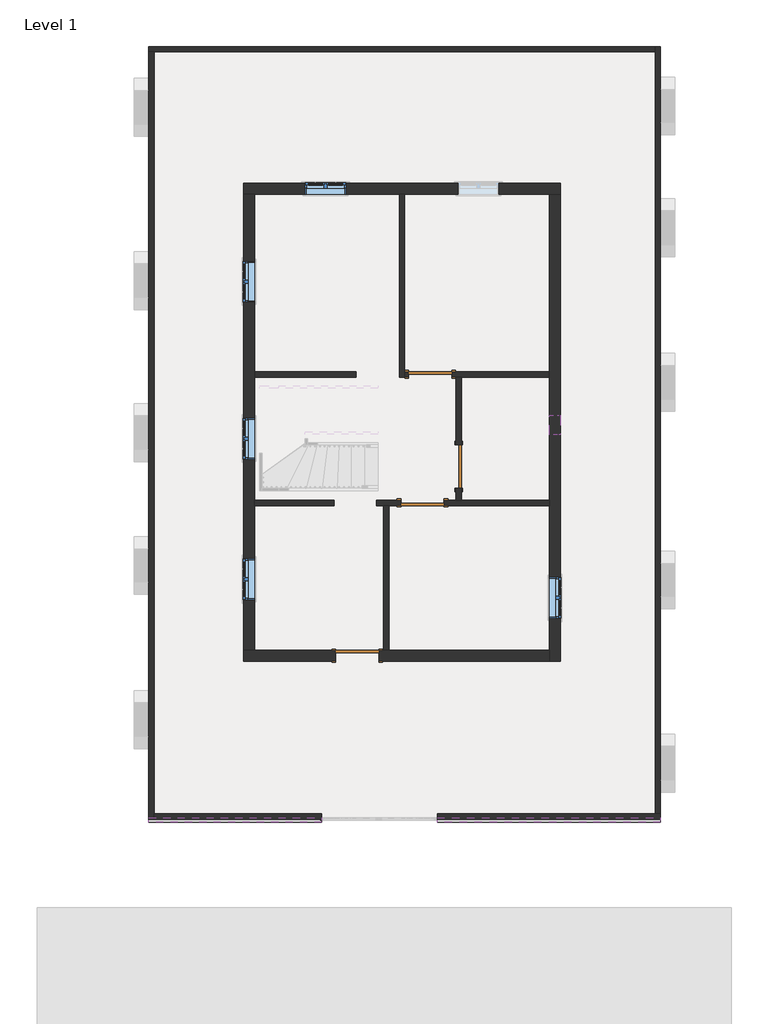
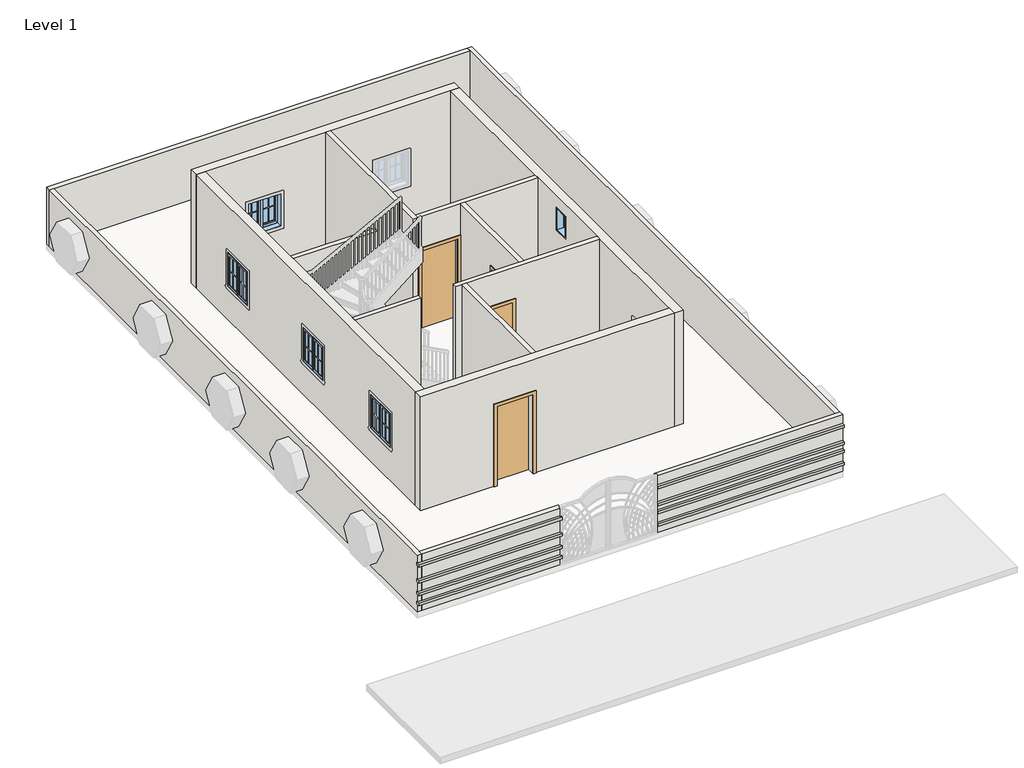
# One storey, part 1 of 3: 16 walls, 8 proxies, 6 windows, 4 doors.
"""IFC4 building model written with IfcOpenShell, lengths in millimetres."""

from ifc_helpers import new_model, si_unit, frame, origin, origin_with_axes, place, context, project, spatial, polyline, outline, extrude, faceted_brep, transform, mapped, element, save
from components import door_e5f9f3c4, door_305aa2a5, door_a90ba1ad, window_aa618e30, window_339605e1

model = new_model("IFC4")

# Units and contexts
model_context = context("Model", 3, world=origin())
ifc_project = project(units=[si_unit("LENGTHUNIT", "METRE", prefix="MILLI")], contexts=[model_context])

# Site, building, storey
site = spatial("IfcSite", under=ifc_project)
building = spatial("IfcBuilding", under=site)
storey = spatial("IfcBuildingStorey", under=building, Name="Level 1", Elevation=0.0)

# Proxies
placement = place(None, origin())
element("IfcBuildingElementProxy", 1, Name="Reveal", ObjectType="Reveal", at=placement, inside=storey, context=model_context, shape_type="SweptSolid", body=[
    extrude(outline(polyline([(-2968.1372391, -8199.8056704), (-2968.1372391, -8291.8806704), (-6606.6872391, -8291.8806704), (-6606.6872391, -8199.8056704), (-2968.1372391, -8199.8056704)])), frame((0.0, 0.0, 1244.6), z_axis=(0.0, 0.0, 1.0), x_axis=(1.0, 0.0, 0.0)), (0.0, 0.0, 1.0), 67.7333333),
])
element("IfcBuildingElementProxy", 2, Name="Reveal", ObjectType="Reveal", at=placement, inside=storey, context=model_context, shape_type="SweptSolid", body=[
    extrude(outline(polyline([(-2968.1372391, -8199.8056704), (-2968.1372391, -8291.8806704), (-6606.6872391, -8291.8806704), (-6606.6872391, -8199.8056704), (-2968.1372391, -8199.8056704)])), frame((0.0, 0.0, 811.8306593), z_axis=(0.0, 0.0, 1.0), x_axis=(1.0, 0.0, 0.0)), (0.0, 0.0, 1.0), 67.7333333),
])
element("IfcBuildingElementProxy", 3, Name="Reveal", ObjectType="Reveal", at=placement, inside=storey, context=model_context, shape_type="SweptSolid", body=[
    extrude(outline(polyline([(-2968.1372391, -8199.8056704), (-2968.1372391, -8291.8806704), (-6606.6872391, -8291.8806704), (-6606.6872391, -8199.8056704), (-2968.1372391, -8199.8056704)])), frame((0.0, 0.0, 475.0919078), z_axis=(0.0, 0.0, 1.0), x_axis=(1.0, 0.0, 0.0)), (0.0, 0.0, 1.0), 67.7333333),
])
element("IfcBuildingElementProxy", 4, Name="Reveal", ObjectType="Reveal", at=placement, inside=storey, context=model_context, shape_type="SweptSolid", body=[
    extrude(outline(polyline([(-2968.1372391, -8199.8056704), (-2968.1372391, -8291.8806704), (-6606.6872391, -8291.8806704), (-6606.6872391, -8199.8056704), (-2968.1372391, -8199.8056704)])), frame((0.0, 0.0, 205.7009067), z_axis=(0.0, 0.0, 1.0), x_axis=(1.0, 0.0, 0.0)), (0.0, 0.0, 1.0), 67.7333333),
])
element("IfcBuildingElementProxy", 5, Name="Reveal", ObjectType="Reveal", at=placement, inside=storey, context=model_context, shape_type="SweptSolid", body=[
    extrude(outline(polyline([(4175.6127609, -8199.8056704), (4175.6127609, -8291.8806704), (-529.7372391, -8291.8806704), (-529.7372391, -8199.8056704), (4175.6127609, -8199.8056704)])), frame((0.0, 0.0, 1219.2), z_axis=(0.0, 0.0, 1.0), x_axis=(1.0, 0.0, 0.0)), (0.0, 0.0, 1.0), 67.7333333),
])
element("IfcBuildingElementProxy", 6, Name="Reveal", ObjectType="Reveal", at=placement, inside=storey, context=model_context, shape_type="SweptSolid", body=[
    extrude(outline(polyline([(4175.6127609, -8199.8056704), (4175.6127609, -8291.8806704), (-529.7372391, -8291.8806704), (-529.7372391, -8199.8056704), (4175.6127609, -8199.8056704)])), frame((0.0, 0.0, 763.331691), z_axis=(0.0, 0.0, 1.0), x_axis=(1.0, 0.0, 0.0)), (0.0, 0.0, 1.0), 67.7333333),
])
element("IfcBuildingElementProxy", 7, Name="Reveal", ObjectType="Reveal", at=placement, inside=storey, context=model_context, shape_type="SweptSolid", body=[
    extrude(outline(polyline([(4175.6127609, -8199.8056704), (4175.6127609, -8291.8806704), (-529.7372391, -8291.8806704), (-529.7372391, -8199.8056704), (4175.6127609, -8199.8056704)])), frame((0.0, 0.0, 545.0675235), z_axis=(0.0, 0.0, 1.0), x_axis=(1.0, 0.0, 0.0)), (0.0, 0.0, 1.0), 67.7333333),
])
element("IfcBuildingElementProxy", 8, Name="Reveal", ObjectType="Reveal", at=placement, inside=storey, context=model_context, shape_type="SweptSolid", body=[
    extrude(outline(polyline([(4175.6127609, -8199.8056704), (4175.6127609, -8291.8806704), (-529.7372391, -8291.8806704), (-529.7372391, -8199.8056704), (4175.6127609, -8199.8056704)])), frame((0.0, 0.0, 208.3287721), z_axis=(0.0, 0.0, 1.0), x_axis=(1.0, 0.0, 0.0)), (0.0, 0.0, 1.0), 67.7333333),
])

# Doors
door_shape = door_e5f9f3c4(model_context)
element("IfcDoor", 9, ObjectType="Single-Flush : 36\" x 84\"", at=placement, inside=storey, context=model_context, shape_type="MappedRepresentation", body=[
    mapped(door_shape, transform((-78.9949167, -802.9070853, 0.0), x_axis=(0.0, -1.0, 0.0), y_axis=(1.0, 0.0, 0.0), z_axis=(0.0, 0.0, 1.0))),
])
element("IfcDoor", 10, ObjectType="Single-Flush : 36\" x 84\"", at=placement, inside=storey, context=model_context, shape_type="MappedRepresentation", body=[
    mapped(door_shape, transform((-840.9949167, -1564.9070853, 0.0), x_axis=(-1.0, 0.0, 0.0), y_axis=(0.0, -1.0, 0.0), z_axis=(0.0, 0.0, 1.0))),
])
door_2_shape = door_305aa2a5(model_context)
element("IfcDoor", 11, ObjectType="Single-Flush : 36\" x 84\"", at=placement, inside=storey, context=model_context, shape_type="MappedRepresentation", body=[
    mapped(door_2_shape, transform((-675.8949167, 1140.1929147, 0.0), x_axis=(-1.0, 0.0, 0.0), y_axis=(0.0, -1.0, 0.0), z_axis=(0.0, 0.0, 1.0))),
])
door_3_shape = door_a90ba1ad(model_context)
element("IfcDoor", 12, ObjectType="Single-Flush : 36\" x 84\"", at=placement, inside=storey, context=model_context, shape_type="MappedRepresentation", body=[
    mapped(door_3_shape, transform((-2212.5949167, -4784.3570853, 0.0), x_axis=(-1.0, 0.0, 0.0), y_axis=(0.0, -1.0, 0.0), z_axis=(0.0, 0.0, 1.0))),
])

# Walls
element("IfcWall", 13, ObjectType="WALL4.5\"", at=placement, inside=storey, context=model_context, shape_type="Brep", body=[
    faceted_brep([(-1329.9449167, 4931.1429147, 0.0), (-1329.9449167, 1083.0429147, 0.0), (-1329.9449167, 1083.0429147, 3048.0), (-1329.9449167, 4931.1429147, 3048.0), (-1215.6449167, 4931.1429147, 0.0), (-1215.6449167, 4931.1429147, 3048.0), (-1215.6449167, 1197.3429147, 3048.0), (-1215.6449167, 1083.0429147, 3048.0), (-1215.6449167, 1083.0429147, 0.0), (-1215.6449167, 1197.3429147, 0.0)], [[[0, 1, 2, 3]], [[4, 5, 6, 7, 8, 9]], [[1, 0, 4, 9, 8]], [[0, 3, 5, 4]], [[2, 1, 8, 7]], [[3, 2, 7, 6, 5]]]),
])
element("IfcWall", 14, ObjectType="WALL4.5\"", at=placement, inside=storey, context=model_context, shape_type="Brep", body=[
    faceted_brep([(-1215.6449167, 1083.0429147, 0.0), (-1133.0949167, 1083.0429147, 0.0), (-1133.0949167, 1083.0429147, 2133.6), (-218.6949167, 1083.0429147, 2133.6), (-218.6949167, 1083.0429147, 0.0), (-136.1449167, 1083.0429147, 0.0), (-21.8449167, 1083.0429147, 0.0), (1832.3550833, 1083.0429147, 0.0), (1832.3550833, 1083.0429147, 3048.0), (-21.8449167, 1083.0429147, 3048.0), (-136.1449167, 1083.0429147, 3048.0), (-1215.6449167, 1083.0429147, 3048.0), (-1133.0949167, 1197.3429147, 2133.6), (-1133.0949167, 1197.3429147, 0.0), (-1215.6449167, 1197.3429147, 0.0), (-1215.6449167, 1197.3429147, 3048.0), (1832.3550833, 1197.3429147, 3048.0), (1832.3550833, 1197.3429147, 0.0), (-218.6949167, 1197.3429147, 0.0), (-218.6949167, 1197.3429147, 2133.6)], [[[0, 1, 2, 3, 4, 5, 6, 7, 8, 9, 10, 11]], [[12, 13, 14, 15, 16, 17, 18, 19]], [[18, 17, 7, 6, 5, 4]], [[14, 13, 1, 0]], [[0, 11, 15, 14]], [[8, 7, 17, 16]], [[2, 1, 13, 12]], [[3, 2, 12, 19]], [[4, 3, 19, 18]], [[11, 10, 9, 8, 16, 15]]]),
])
element("IfcWall", 15, ObjectType="WALL4.5\"", at=placement, inside=storey, context=model_context, shape_type="SweptSolid", body=[
    extrude(outline(polyline([(-2244.3449167, 1083.0429147), (-4377.9449167, 1083.0429147), (-4377.9449167, 1197.3429147), (-2244.3449167, 1197.3429147), (-2244.3449167, 1083.0429147)])), origin_with_axes(), (0.0, 0.0, 1.0), 3048.0),
])
element("IfcWall", 16, ObjectType="WALL4.5\"", at=placement, inside=storey, context=model_context, shape_type="SweptSolid", body=[
    extrude(outline(polyline([(-1260.1070853, 2133.6), (-1260.1070853, 0.0), (-1507.7570853, 0.0), (-1507.7570853, 3048.0), (1083.0429147, 3048.0), (1083.0429147, 0.0), (-345.7070853, 0.0), (-345.7070853, 2133.6), (-1260.1070853, 2133.6)])), frame((-136.1449167, 0.0, 0.0), z_axis=(1.0, 0.0, 0.0), x_axis=(0.0, 1.0, 0.0)), (0.0, 0.0, 1.0), 114.3),
])
element("IfcWall", 17, ObjectType="WALL4.5\"", at=placement, inside=storey, context=model_context, shape_type="SweptSolid", body=[
    extrude(outline(polyline([(-2701.5449167, -1622.0570853), (-4377.9449167, -1622.0570853), (-4377.9449167, -1507.7570853), (-2701.5449167, -1507.7570853), (-2701.5449167, -1622.0570853)])), origin_with_axes(), (0.0, 0.0, 1.0), 3048.0),
])
element("IfcWall", 18, ObjectType="WALL4.5\"", at=placement, inside=storey, context=model_context, shape_type="Brep", body=[
    faceted_brep([(-1812.5449167, -1622.0570853, 0.0), (-1660.1449167, -1622.0570853, 0.0), (-1545.8449167, -1622.0570853, 0.0), (-1298.1949167, -1622.0570853, 0.0), (-1298.1949167, -1622.0570853, 2133.6), (-383.7949167, -1622.0570853, 2133.6), (-383.7949167, -1622.0570853, 0.0), (1832.3550833, -1622.0570853, 0.0), (1832.3550833, -1622.0570853, 3048.0), (-1545.8449167, -1622.0570853, 3048.0), (-1660.1449167, -1622.0570853, 3048.0), (-1812.5449167, -1622.0570853, 3048.0), (-1298.1949167, -1507.7570853, 2133.6), (-1298.1949167, -1507.7570853, 0.0), (-1812.5449167, -1507.7570853, 0.0), (-1812.5449167, -1507.7570853, 3048.0), (-136.1449167, -1507.7570853, 3048.0), (-21.8449167, -1507.7570853, 3048.0), (1832.3550833, -1507.7570853, 3048.0), (1832.3550833, -1507.7570853, 0.0), (-21.8449167, -1507.7570853, 0.0), (-136.1449167, -1507.7570853, 0.0), (-383.7949167, -1507.7570853, 0.0), (-383.7949167, -1507.7570853, 2133.6)], [[[0, 1, 2, 3, 4, 5, 6, 7, 8, 9, 10, 11]], [[12, 13, 14, 15, 16, 17, 18, 19, 20, 21, 22, 23]], [[14, 13, 3, 2, 1, 0]], [[22, 21, 20, 19, 7, 6]], [[0, 11, 15, 14]], [[8, 7, 19, 18]], [[4, 3, 13, 12]], [[5, 4, 12, 23]], [[6, 5, 23, 22]], [[11, 10, 9, 8, 18, 17, 16, 15]]]),
])
element("IfcWall", 19, ObjectType="WALL4.5\"", at=placement, inside=storey, context=model_context, shape_type="SweptSolid", body=[
    extrude(outline(polyline([(-1660.1449167, -4670.0570853), (-1660.1449167, -1622.0570853), (-1545.8449167, -1622.0570853), (-1545.8449167, -4670.0570853), (-1660.1449167, -4670.0570853)])), origin_with_axes(), (0.0, 0.0, 1.0), 3048.0),
])
element("IfcWall", 20, ObjectType="WALL4.5\"", at=placement, inside=storey, context=model_context, shape_type="Brep", body=[
    faceted_brep([(-6606.6872391, 7929.1943296, 0.0), (-6492.3872391, 7929.1943296, 0.0), (4061.3127609, 7929.1943296, 0.0), (4061.3127609, 7929.1943296, 1524.0), (-6492.3872391, 7929.1943296, 1524.0), (-6606.6872391, 7929.1943296, 1524.0), (-6606.6872391, 8043.4943296, 0.0), (-6606.6872391, 8043.4943296, 1524.0), (4061.3127609, 8043.4943296, 1524.0), (4061.3127609, 8043.4943296, 0.0)], [[[0, 1, 2, 3, 4, 5]], [[6, 7, 8, 9]], [[2, 1, 0, 6, 9]], [[5, 4, 3, 8, 7]], [[0, 5, 7, 6]], [[3, 2, 9, 8]]]),
])
element("IfcWall", 21, ObjectType="WALL4.5\"", at=placement, inside=storey, context=model_context, shape_type="Brep", body=[
    faceted_brep([(-6492.3872391, -8225.2056704, 0.0), (-6492.3872391, -8110.9056704, 0.0), (-6492.3872391, 7929.1943296, 0.0), (-6492.3872391, 7929.1943296, 1524.0), (-6492.3872391, -8110.9056704, 1524.0), (-6492.3872391, -8225.2056704, 1524.0), (-6492.3872391, -8225.2056704, 1312.3333333), (-6492.3872391, -8199.8056704, 1312.3333333), (-6492.3872391, -8199.8056704, 1244.6), (-6492.3872391, -8225.2056704, 1244.6), (-6492.3872391, -8225.2056704, 879.5639926), (-6492.3872391, -8199.8056704, 879.5639926), (-6492.3872391, -8199.8056704, 811.8306593), (-6492.3872391, -8225.2056704, 811.8306593), (-6492.3872391, -8225.2056704, 542.8252412), (-6492.3872391, -8199.8056704, 542.8252412), (-6492.3872391, -8199.8056704, 475.0919078), (-6492.3872391, -8225.2056704, 475.0919078), (-6492.3872391, -8225.2056704, 273.43424), (-6492.3872391, -8199.8056704, 273.43424), (-6492.3872391, -8199.8056704, 205.7009067), (-6492.3872391, -8225.2056704, 205.7009067), (-6606.6872391, 7929.1943296, 0.0), (-6606.6872391, -8225.2056704, 0.0), (-6606.6872391, -8225.2056704, 205.7009067), (-6606.6872391, -8199.8056704, 205.7009067), (-6606.6872391, -8199.8056704, 273.43424), (-6606.6872391, -8225.2056704, 273.43424), (-6606.6872391, -8225.2056704, 475.0919078), (-6606.6872391, -8199.8056704, 475.0919078), (-6606.6872391, -8199.8056704, 542.8252412), (-6606.6872391, -8225.2056704, 542.8252412), (-6606.6872391, -8225.2056704, 811.8306593), (-6606.6872391, -8199.8056704, 811.8306593), (-6606.6872391, -8199.8056704, 879.5639926), (-6606.6872391, -8225.2056704, 879.5639926), (-6606.6872391, -8225.2056704, 1244.6), (-6606.6872391, -8199.8056704, 1244.6), (-6606.6872391, -8199.8056704, 1312.3333333), (-6606.6872391, -8225.2056704, 1312.3333333), (-6606.6872391, -8225.2056704, 1524.0), (-6606.6872391, 7929.1943296, 1524.0)], [[[0, 1, 2, 3, 4, 5, 6, 7, 8, 9, 10, 11, 12, 13, 14, 15, 16, 17, 18, 19, 20, 21]], [[22, 23, 24, 25, 26, 27, 28, 29, 30, 31, 32, 33, 34, 35, 36, 37, 38, 39, 40, 41]], [[2, 1, 0, 23, 22]], [[5, 4, 3, 41, 40]], [[5, 40, 39, 6]], [[23, 0, 21, 24]], [[9, 36, 35, 10]], [[13, 32, 31, 14]], [[17, 28, 27, 18]], [[3, 2, 22, 41]], [[38, 7, 6, 39]], [[8, 37, 36, 9]], [[7, 38, 37, 8]], [[34, 11, 10, 35]], [[12, 33, 32, 13]], [[11, 34, 33, 12]], [[30, 15, 14, 31]], [[16, 29, 28, 17]], [[15, 30, 29, 16]], [[26, 19, 18, 27]], [[20, 25, 24, 21]], [[19, 26, 25, 20]]]),
])
element("IfcWall", 22, ObjectType="WALL4.5\"", at=placement, inside=storey, context=model_context, shape_type="Brep", body=[
    faceted_brep([(4175.6127609, -8110.9056704, 0.0), (4061.3127609, -8110.9056704, 0.0), (-529.7372391, -8110.9056704, 0.0), (-529.7372391, -8110.9056704, 1524.0), (4061.3127609, -8110.9056704, 1524.0), (4175.6127609, -8110.9056704, 1524.0), (-529.7372391, -8225.2056704, 0.0), (4175.6127609, -8225.2056704, 0.0), (4175.6127609, -8225.2056704, 208.3287721), (-529.7372391, -8225.2056704, 208.3287721), (4175.6127609, -8225.2056704, 1524.0), (-529.7372391, -8225.2056704, 1524.0), (-529.7372391, -8225.2056704, 1286.9333333), (4175.6127609, -8225.2056704, 1286.9333333), (4175.6127609, -8225.2056704, 1219.2), (-529.7372391, -8225.2056704, 1219.2), (-529.7372391, -8225.2056704, 831.0650243), (4175.6127609, -8225.2056704, 831.0650243), (4175.6127609, -8225.2056704, 763.331691), (-529.7372391, -8225.2056704, 763.331691), (-529.7372391, -8225.2056704, 612.8008568), (4175.6127609, -8225.2056704, 612.8008568), (4175.6127609, -8225.2056704, 545.0675235), (-529.7372391, -8225.2056704, 545.0675235), (-529.7372391, -8225.2056704, 276.0621054), (4175.6127609, -8225.2056704, 276.0621054), (-529.7372391, -8199.8056704, 208.3287721), (-529.7372391, -8199.8056704, 276.0621054), (-529.7372391, -8199.8056704, 545.0675235), (-529.7372391, -8199.8056704, 612.8008568), (-529.7372391, -8199.8056704, 763.331691), (-529.7372391, -8199.8056704, 831.0650243), (-529.7372391, -8199.8056704, 1219.2), (-529.7372391, -8199.8056704, 1286.9333333), (4175.6127609, -8199.8056704, 1286.9333333), (4175.6127609, -8199.8056704, 1219.2), (4175.6127609, -8199.8056704, 831.0650243), (4175.6127609, -8199.8056704, 763.331691), (4175.6127609, -8199.8056704, 612.8008568), (4175.6127609, -8199.8056704, 545.0675235), (4175.6127609, -8199.8056704, 276.0621054), (4175.6127609, -8199.8056704, 208.3287721)], [[[0, 1, 2, 3, 4, 5]], [[6, 7, 8, 9]], [[10, 11, 12, 13]], [[14, 15, 16, 17]], [[18, 19, 20, 21]], [[22, 23, 24, 25]], [[2, 1, 0, 7, 6]], [[3, 2, 6, 9, 26, 27, 24, 23, 28, 29, 20, 19, 30, 31, 16, 15, 32, 33, 12, 11]], [[5, 4, 3, 11, 10]], [[0, 5, 10, 13, 34, 35, 14, 17, 36, 37, 18, 21, 38, 39, 22, 25, 40, 41, 8, 7]], [[33, 34, 13, 12]], [[35, 32, 15, 14]], [[34, 33, 32, 35]], [[31, 36, 17, 16]], [[37, 30, 19, 18]], [[36, 31, 30, 37]], [[29, 38, 21, 20]], [[39, 28, 23, 22]], [[38, 29, 28, 39]], [[27, 40, 25, 24]], [[41, 26, 9, 8]], [[40, 27, 26, 41]]]),
])
element("IfcWall", 23, ObjectType="WALL4.5\"", at=placement, inside=storey, context=model_context, shape_type="Brep", body=[
    faceted_brep([(4061.3127609, 8043.4943296, 0.0), (4061.3127609, 7929.1943296, 0.0), (4061.3127609, -8110.9056704, 0.0), (4061.3127609, -8110.9056704, 1524.0), (4061.3127609, 7929.1943296, 1524.0), (4061.3127609, 8043.4943296, 1524.0), (4175.6127609, 8043.4943296, 0.0), (4175.6127609, 8043.4943296, 1524.0), (4175.6127609, -8110.9056704, 1524.0), (4175.6127609, -8110.9056704, 0.0)], [[[0, 1, 2, 3, 4, 5]], [[6, 7, 8, 9]], [[2, 1, 0, 6, 9]], [[5, 4, 3, 8, 7]], [[0, 5, 7, 6]], [[3, 2, 9, 8]]]),
])
element("IfcWall", 24, ObjectType="WALL4.5\"", at=placement, inside=storey, context=model_context, shape_type="SweptSolid", body=[
    extrude(outline(polyline([(-8110.9056704, 1524.0), (-8110.9056704, 0.0), (-8225.2056704, 0.0), (-8225.2056704, 205.7009067), (-8199.8056704, 205.7009067), (-8199.8056704, 273.43424), (-8225.2056704, 273.43424), (-8225.2056704, 475.0919078), (-8199.8056704, 475.0919078), (-8199.8056704, 542.8252412), (-8225.2056704, 542.8252412), (-8225.2056704, 811.8306593), (-8199.8056704, 811.8306593), (-8199.8056704, 879.5639926), (-8225.2056704, 879.5639926), (-8225.2056704, 1244.6), (-8199.8056704, 1244.6), (-8199.8056704, 1312.3333333), (-8225.2056704, 1312.3333333), (-8225.2056704, 1524.0), (-8110.9056704, 1524.0)])), frame((-6492.3872391, 0.0, 0.0), z_axis=(1.0, 0.0, 0.0), x_axis=(0.0, 1.0, 0.0)), (0.0, 0.0, 1.0), 3524.25),
])
element("IfcWall", 25, ObjectType="WALL9\"", at=placement, inside=storey, context=model_context, shape_type="Brep", body=[
    faceted_brep([(-4606.5449167, 4931.1429147, 0.0), (-4377.9449167, 4931.1429147, 0.0), (-1329.9449167, 4931.1429147, 0.0), (-1215.6449167, 4931.1429147, 0.0), (1832.3550833, 4931.1429147, 0.0), (2060.9550833, 4931.1429147, 0.0), (2060.9550833, 4931.1429147, 3048.0), (1832.3550833, 4931.1429147, 3048.0), (-1215.6449167, 4931.1429147, 3048.0), (-1329.9449167, 4931.1429147, 3048.0), (-4377.9449167, 4931.1429147, 3048.0), (-4606.5449167, 4931.1429147, 3048.0), (-2450.7199167, 4931.1429147, 1828.8), (-2450.7199167, 4931.1429147, 914.4), (-3314.3199167, 4931.1429147, 914.4), (-3314.3199167, 4931.1429147, 1828.8), (768.7300833, 4931.1429147, 1828.8), (768.7300833, 4931.1429147, 914.4), (-94.8699167, 4931.1429147, 914.4), (-94.8699167, 4931.1429147, 1828.8), (-4606.5449167, 5159.7429147, 0.0), (-4606.5449167, 5159.7429147, 3048.0), (2060.9550833, 5159.7429147, 3048.0), (2060.9550833, 5159.7429147, 0.0), (-2450.7199167, 5159.7429147, 1828.8), (-3314.3199167, 5159.7429147, 1828.8), (-3314.3199167, 5159.7429147, 914.4), (-2450.7199167, 5159.7429147, 914.4), (768.7300833, 5159.7429147, 1828.8), (-94.8699167, 5159.7429147, 1828.8), (-94.8699167, 5159.7429147, 914.4), (768.7300833, 5159.7429147, 914.4)], [[[0, 1, 2, 3, 4, 5, 6, 7, 8, 9, 10, 11], [12, 13, 14, 15], [16, 17, 18, 19]], [[20, 21, 22, 23], [24, 25, 26, 27], [28, 29, 30, 31]], [[5, 4, 3, 2, 1, 0, 20, 23]], [[6, 5, 23, 22]], [[0, 11, 21, 20]], [[11, 10, 9, 8, 7, 6, 22, 21]], [[13, 12, 24, 27]], [[14, 13, 27, 26]], [[15, 14, 26, 25]], [[12, 15, 25, 24]], [[17, 16, 28, 31]], [[18, 17, 31, 30]], [[19, 18, 30, 29]], [[16, 19, 29, 28]]]),
])
element("IfcWall", 26, ObjectType="WALL9\"", at=placement, inside=storey, context=model_context, shape_type="Brep", body=[
    faceted_brep([(1832.3550833, 4931.1429147, 0.0), (1832.3550833, 1197.3429147, 0.0), (1832.3550833, 1083.0429147, 0.0), (1832.3550833, -1507.7570853, 0.0), (1832.3550833, -1622.0570853, 0.0), (1832.3550833, -4670.0570853, 0.0), (1832.3550833, -4898.6570853, 0.0), (1832.3550833, -4898.6570853, 3048.0), (1832.3550833, -4670.0570853, 3048.0), (1832.3550833, -1622.0570853, 3048.0), (1832.3550833, -1507.7570853, 3048.0), (1832.3550833, 1083.0429147, 3048.0), (1832.3550833, 1197.3429147, 3048.0), (1832.3550833, 4931.1429147, 3048.0), (1832.3550833, -129.8070853, 2743.2), (1832.3550833, -129.8070853, 2133.6), (1832.3550833, 276.5929147, 2133.6), (1832.3550833, 276.5929147, 2743.2), (1832.3550833, -3996.9570853, 1828.8), (1832.3550833, -3996.9570853, 914.4), (1832.3550833, -3133.3570853, 914.4), (1832.3550833, -3133.3570853, 1828.8), (2060.9550833, 4931.1429147, 0.0), (2060.9550833, 4931.1429147, 3048.0), (2060.9550833, -4898.6570853, 3048.0), (2060.9550833, -4898.6570853, 0.0), (2060.9550833, -129.8070853, 2743.2), (2060.9550833, 276.5929147, 2743.2), (2060.9550833, 276.5929147, 2133.6), (2060.9550833, -129.8070853, 2133.6), (2060.9550833, -3996.9570853, 1828.8), (2060.9550833, -3133.3570853, 1828.8), (2060.9550833, -3133.3570853, 914.4), (2060.9550833, -3996.9570853, 914.4)], [[[0, 1, 2, 3, 4, 5, 6, 7, 8, 9, 10, 11, 12, 13], [14, 15, 16, 17], [18, 19, 20, 21]], [[22, 23, 24, 25], [26, 27, 28, 29], [30, 31, 32, 33]], [[6, 5, 4, 3, 2, 1, 0, 22, 25]], [[0, 13, 23, 22]], [[7, 6, 25, 24]], [[13, 12, 11, 10, 9, 8, 7, 24, 23]], [[15, 14, 26, 29]], [[16, 15, 29, 28]], [[17, 16, 28, 27]], [[14, 17, 27, 26]], [[19, 18, 30, 33]], [[20, 19, 33, 32]], [[21, 20, 32, 31]], [[18, 21, 31, 30]]]),
])
element("IfcWall", 27, ObjectType="WALL9\"", at=placement, inside=storey, context=model_context, shape_type="Brep", body=[
    faceted_brep([(-2669.7949167, -4670.0570853, 2133.6), (-2669.7949167, -4670.0570853, 0.0), (-4377.9449167, -4670.0570853, 0.0), (-4606.5449167, -4670.0570853, 0.0), (-4606.5449167, -4670.0570853, 3048.0), (-4377.9449167, -4670.0570853, 3048.0), (-1660.1449167, -4670.0570853, 3048.0), (-1545.8449167, -4670.0570853, 3048.0), (1832.3550833, -4670.0570853, 3048.0), (1832.3550833, -4670.0570853, 0.0), (-1545.8449167, -4670.0570853, 0.0), (-1660.1449167, -4670.0570853, 0.0), (-1755.3949167, -4670.0570853, 0.0), (-1755.3949167, -4670.0570853, 2133.6), (-4606.5449167, -4898.6570853, 0.0), (-2669.7949167, -4898.6570853, 0.0), (-2669.7949167, -4898.6570853, 2133.6), (-1755.3949167, -4898.6570853, 2133.6), (-1755.3949167, -4898.6570853, 0.0), (1832.3550833, -4898.6570853, 0.0), (1832.3550833, -4898.6570853, 2590.8), (1832.3550833, -4898.6570853, 2658.5333333), (1832.3550833, -4898.6570853, 3048.0), (-4606.5449167, -4898.6570853, 3048.0)], [[[0, 1, 2, 3, 4, 5, 6, 7, 8, 9, 10, 11, 12, 13]], [[14, 15, 16, 17, 18, 19, 20, 21, 22, 23]], [[3, 2, 1, 15, 14]], [[12, 11, 10, 9, 19, 18]], [[9, 8, 22, 21, 20, 19]], [[4, 3, 14, 23]], [[16, 15, 1, 0]], [[17, 16, 0, 13]], [[18, 17, 13, 12]], [[8, 7, 6, 5, 4, 23, 22]]]),
])
element("IfcWall", 28, ObjectType="WALL9\"", at=placement, inside=storey, context=model_context, shape_type="Brep", body=[
    faceted_brep([(-4377.9449167, -4670.0570853, 0.0), (-4377.9449167, -1622.0570853, 0.0), (-4377.9449167, -1507.7570853, 0.0), (-4377.9449167, 1083.0429147, 0.0), (-4377.9449167, 1197.3429147, 0.0), (-4377.9449167, 4931.1429147, 0.0), (-4377.9449167, 4931.1429147, 3048.0), (-4377.9449167, 1197.3429147, 3048.0), (-4377.9449167, 1083.0429147, 3048.0), (-4377.9449167, -1507.7570853, 3048.0), (-4377.9449167, -1622.0570853, 3048.0), (-4377.9449167, -4670.0570853, 3048.0), (-4377.9449167, 219.4429147, 1828.8), (-4377.9449167, 219.4429147, 914.4), (-4377.9449167, -644.1570853, 914.4), (-4377.9449167, -644.1570853, 1828.8), (-4377.9449167, -2742.8320853, 1828.8), (-4377.9449167, -2742.8320853, 914.4), (-4377.9449167, -3606.4320853, 914.4), (-4377.9449167, -3606.4320853, 1828.8), (-4377.9449167, 3524.6179147, 1828.8), (-4377.9449167, 3524.6179147, 914.4), (-4377.9449167, 2661.0179147, 914.4), (-4377.9449167, 2661.0179147, 1828.8), (-4606.5449167, -4670.0570853, 0.0), (-4606.5449167, -4670.0570853, 3048.0), (-4606.5449167, 4931.1429147, 3048.0), (-4606.5449167, 4931.1429147, 0.0), (-4606.5449167, 219.4429147, 1828.8), (-4606.5449167, -644.1570853, 1828.8), (-4606.5449167, -644.1570853, 914.4), (-4606.5449167, 219.4429147, 914.4), (-4606.5449167, -2742.8320853, 1828.8), (-4606.5449167, -3606.4320853, 1828.8), (-4606.5449167, -3606.4320853, 914.4), (-4606.5449167, -2742.8320853, 914.4), (-4606.5449167, 3524.6179147, 1828.8), (-4606.5449167, 2661.0179147, 1828.8), (-4606.5449167, 2661.0179147, 914.4), (-4606.5449167, 3524.6179147, 914.4)], [[[0, 1, 2, 3, 4, 5, 6, 7, 8, 9, 10, 11], [12, 13, 14, 15], [16, 17, 18, 19], [20, 21, 22, 23]], [[24, 25, 26, 27], [28, 29, 30, 31], [32, 33, 34, 35], [36, 37, 38, 39]], [[5, 4, 3, 2, 1, 0, 24, 27]], [[0, 11, 25, 24]], [[6, 5, 27, 26]], [[11, 10, 9, 8, 7, 6, 26, 25]], [[13, 12, 28, 31]], [[14, 13, 31, 30]], [[15, 14, 30, 29]], [[12, 15, 29, 28]], [[17, 16, 32, 35]], [[18, 17, 35, 34]], [[19, 18, 34, 33]], [[16, 19, 33, 32]], [[21, 20, 36, 39]], [[22, 21, 39, 38]], [[23, 22, 38, 37]], [[20, 23, 37, 36]]]),
])

# Windows
window_shape = window_aa618e30(model_context)
element("IfcWindow", 29, ObjectType="Fixed : 16\" x 24\"", at=placement, inside=storey, context=model_context, shape_type="MappedRepresentation", body=[
    mapped(window_shape, transform((1946.6550833, 35.2929147, 1219.2), x_axis=(0.0, -1.0, 0.0), y_axis=(1.0, 0.0, 0.0), z_axis=(0.0, 0.0, 1.0))),
])
window_2_shape = window_339605e1(model_context)
element("IfcWindow", 30, ObjectType="Window-Casement-Double : 34\" x 36\"", at=placement, inside=storey, context=model_context, shape_type="MappedRepresentation", body=[
    mapped(window_2_shape, transform((-2882.5199167, 5045.4429147, 0.0), x_axis=(1.0, 0.0, 0.0), y_axis=(0.0, 1.0, 0.0), z_axis=(0.0, 0.0, 1.0))),
])
element("IfcWindow", 31, ObjectType="Window-Casement-Double : 34\" x 36\"", at=placement, inside=storey, context=model_context, shape_type="MappedRepresentation", body=[
    mapped(window_2_shape, transform((1946.6550833, -3565.1570853, 0.0), x_axis=(0.0, -1.0, 0.0), y_axis=(1.0, 0.0, 0.0), z_axis=(0.0, 0.0, 1.0))),
])
element("IfcWindow", 32, ObjectType="Window-Casement-Double : 34\" x 36\"", at=placement, inside=storey, context=model_context, shape_type="MappedRepresentation", body=[
    mapped(window_2_shape, transform((-4492.2449167, -212.3570853, 0.0), x_axis=(0.0, 1.0, 0.0), y_axis=(-1.0, 0.0, 0.0), z_axis=(0.0, 0.0, 1.0))),
])
element("IfcWindow", 33, ObjectType="Window-Casement-Double : 34\" x 36\"", at=placement, inside=storey, context=model_context, shape_type="MappedRepresentation", body=[
    mapped(window_2_shape, transform((-4492.2449167, -3174.6320853, 0.0), x_axis=(0.0, 1.0, 0.0), y_axis=(-1.0, 0.0, 0.0), z_axis=(0.0, 0.0, 1.0))),
])
element("IfcWindow", 34, ObjectType="Window-Casement-Double : 34\" x 36\"", at=placement, inside=storey, context=model_context, shape_type="MappedRepresentation", body=[
    mapped(window_2_shape, transform((-4492.2449167, 3092.8179147, 0.0), x_axis=(0.0, 1.0, 0.0), y_axis=(-1.0, 0.0, 0.0), z_axis=(0.0, 0.0, 1.0))),
])

save(model, "model.ifc")

# Revit data of these elements
# Type "Single-Flush : 36\" x 84\""
#   Type Mark = "1"
#   Construction Type Id = "MDOOR"
#   Assembly Code = "C1020"
#   Analytic Construction = "Metal"
#   Thickness = 0' - 2"
#   Heat Transfer Coefficient (U) = 0.651978 BTU/(h·ft²·°F)
#   Height = 7' - 0"
#   Trim Projection Ext = 0' - 1"
#   Trim Projection Int = 0' - 1"
#   Trim Width = 0' - 3"
#   Width = 3' - 0"
#   Define Thermal Properties by = 1
#   Define Thermal Properties by = 1
#   Door Material = Door - Panel
#   Frame Material = Door - Frame
#   Visual Light Transmittance = 0
#   Solar Heat Gain Coefficient = 0
#   Function = (empty or 0)
#   Wall Closure = (empty or 0)
# Type "WALL4.5\""
#   Assembly Code = "B2010"
#   Layers, outside or top first: 0' - 4 1/2" "Parking Stripe" (function 1)
# Type "WALL9\""
#   Assembly Code = "B2010"
#   Layers, outside or top first: 0' - 9" no material (function 1)
# Type "Fixed : 16\" x 24\""
#   Type Mark = "4"
#   Construction Type Id = "GSP4R"
#   Assembly Code = "B2020100"
#   Analytic Construction = "1/8 in Pilkington single glazing"
#   Visual Light Transmittance = 0.9
#   Solar Heat Gain Coefficient = 0.78
#   Heat Transfer Coefficient (U) = 0.6496 BTU/(h·ft²·°F)
#   Height = 2' - 0"
#   Default Sill Height = 3' - 0"
#   Width = 1' - 4"
#   Window Inset = 0' - 0 3/4"
#   Define Thermal Properties by = 1
#   Define Thermal Properties by = 1
#   Glass Pane Material = Glass
#   Sash Material = Sash
#   Wall Closure = (empty or 0)
# Type "Window-Casement-Double : 34\" x 36\""
#   Type Mark = "14"
#   Fire Rating = "0.5h"
#   Assembly Code = "B2020100"
#   Analytic Construction = "Double glazing - domestic"
#   Frame Extension [instance default] = 0' - 0 1/4"
#   Window Inset [instance default] = 0' - 0"
#   Wall Thickness [instance default] = 0' - 6"
#   Interior Wall Closure [instance default] = 0' - 2 1/4"
#   Half Width = 1' - 5"
#   Visual Light Transmittance = 0.81
#   Thermal Resistance (R) = 1.8146 (h·ft²·°F)/BTU
#   Solar Heat Gain Coefficient = 0.76
#   Rough Width = 2' - 10 1/2"
#   Rough Height = 3' - 0 1/2"
#   Height = 3' - 0"
#   Heat Transfer Coefficient (U) = 0.5511 BTU/(h·ft²·°F)
#   Exterior Wall Closure [instance default] = 0' - 1 1/4"
#   Extension Jamb [instance default] = 0' - 2 1/4"
#   Default Sill Height = 3' - 0"
#   Width = 2' - 10"
#   Define Thermal Properties by = 0
#   Muntin Visibility = yes
#   Interior Trim Visibility [instance default] = yes
#   Exterior Trim Visibility [instance default] = yes
#   Extension Jamb Visibility [instance default] = yes
#   Interior Trim Material = Wood - Stained
#   Muntin Pattern = Muntin Pattern_2x2 : Muntin Pattern_2x2
#   Interior Trim = Trim-Window-Interior-Flat : Picture Frame
#   Interior Frame Material = Wood - Stained
#   Glass Panel Material = Glass
#   Exterior Trim Material = Clad - White
#   Exterior Trim = Trim-Window-Exterior-Flat : with Sill
#   Exterior Frame Material = Clad - White
#   Wall Closure = (empty or 0)
# Elements 9, 10, 11, 12 (IfcDoor, "Single-Flush : 36\" x 84\"")
#   Phase Created = New Construction
#   Materials on its faces: "Door - Frame", "Door - Panel"
# Elements 13, 14, 15, 16, 17, 18, 19 (IfcWall, "WALL4.5\"")
#   Top Offset = 0' - 0"
#   Base Offset = 0' - 0"
#   Unconnected Height = 10' - 0"
#   wall height = 10' - 0"
#   Phase Created = New Construction
#   Base Constraint = Level 1
#   Materials on its faces: "Parking Stripe"
# Elements 20, 21, 22, 23, 24 (IfcWall, "WALL4.5\"")
#   Top Offset = 0' - 0"
#   Base Offset = 0' - 0"
#   Unconnected Height = 5' - 0"
#   wall height = 5' - 0"
#   Phase Created = New Construction
#   Base Constraint = Level 1
#   Materials on its faces: "Parking Stripe", "Brick, Common"
# Elements 25, 26, 27, 28 (IfcWall, "WALL9\"")
#   Top Offset = 0' - 0"
#   Base Offset = 0' - 0"
#   Unconnected Height = 10' - 0"
#   wall height = 10' - 0"
#   Phase Created = New Construction
#   Base Constraint = Level 1
#   Materials on its faces: "Default Wall", "Wood Planks"
# Element 29 (IfcWindow, "Fixed : 16\" x 24\"")
#   Mark = "1"
#   Phase Created = New Construction
#   Materials on its faces: "Sash", "Glass"
# Element 30 (IfcWindow, "Window-Casement-Double : 34\" x 36\"")
#   Mark = "2"
#   Window Inset = 0' - 0"
#   Interior Wall Closure = 0' - 2 1/4"
#   Frame Extension = 0' - 0 1/4"
#   Exterior Wall Closure = 0' - 1 1/4"
#   Interior Trim Visibility = yes
#   Exterior Trim Visibility = yes
#   Phase Created = New Construction
#   Materials on its faces: "Wood - Stained", "Glass", "Clad - White"
# Element 31 (IfcWindow, "Window-Casement-Double : 34\" x 36\"")
#   Mark = "4"
#   Window Inset = 0' - 0"
#   Interior Wall Closure = 0' - 2 1/4"
#   Frame Extension = 0' - 0 1/4"
#   Exterior Wall Closure = 0' - 1 1/4"
#   Interior Trim Visibility = yes
#   Exterior Trim Visibility = yes
#   Phase Created = New Construction
#   Materials on its faces: "Wood - Stained", "Glass", "Clad - White"
# Element 32 (IfcWindow, "Window-Casement-Double : 34\" x 36\"")
#   Mark = "6"
#   Window Inset = 0' - 0"
#   Interior Wall Closure = 0' - 2 1/4"
#   Frame Extension = 0' - 0 1/4"
#   Exterior Wall Closure = 0' - 1 1/4"
#   Interior Trim Visibility = yes
#   Exterior Trim Visibility = yes
#   Phase Created = New Construction
#   Materials on its faces: "Wood - Stained", "Glass", "Clad - White"
# Element 33 (IfcWindow, "Window-Casement-Double : 34\" x 36\"")
#   Mark = "7"
#   Window Inset = 0' - 0"
#   Interior Wall Closure = 0' - 2 1/4"
#   Frame Extension = 0' - 0 1/4"
#   Exterior Wall Closure = 0' - 1 1/4"
#   Interior Trim Visibility = yes
#   Exterior Trim Visibility = yes
#   Phase Created = New Construction
#   Materials on its faces: "Wood - Stained", "Glass", "Clad - White"
# Element 34 (IfcWindow, "Window-Casement-Double : 34\" x 36\"")
#   Mark = "8"
#   Window Inset = 0' - 0"
#   Interior Wall Closure = 0' - 2 1/4"
#   Frame Extension = 0' - 0 1/4"
#   Exterior Wall Closure = 0' - 1 1/4"
#   Interior Trim Visibility = yes
#   Exterior Trim Visibility = yes
#   Phase Created = New Construction
#   Materials on its faces: "Wood - Stained", "Glass", "Clad - White"
# Materials
#   "Door - Panel": class "Wood", colour RGB 210 159 95, transparency 0, Cost = 0
#   "Door - Frame": colour RGB 118 70 51, transparency 0, Cost = 0
#   "Parking Stripe": class "Paint", colour RGB 250 250 91, transparency 0, Cost = 0
#   "Glass": class "Glass", colour RGB 0 128 192, transparency 0.75, Description = "Soda Lime Glass", Cost = 0
#   "Sash": class "Wood", colour RGB 224 178 126, transparency 0, Cost = 0
#   "Wood - Stained": class "Wood", colour RGB 224 178 126, transparency 0, Cost = 0
#   "Clad - White": class "Wood", colour RGB 242 242 238, transparency 0, Cost = 0
#   "Brick, Common": class "Masonry", colour RGB 170 98 104, transparency 0, Description = "Common brick", Cost = 0
#   "Default Wall": colour RGB 128 128 128, transparency 0, Cost = 0
#   "Wood Planks": class "Wood", colour RGB 193 160 115, transparency 0, Description = "Physical material.", Cost = 0
